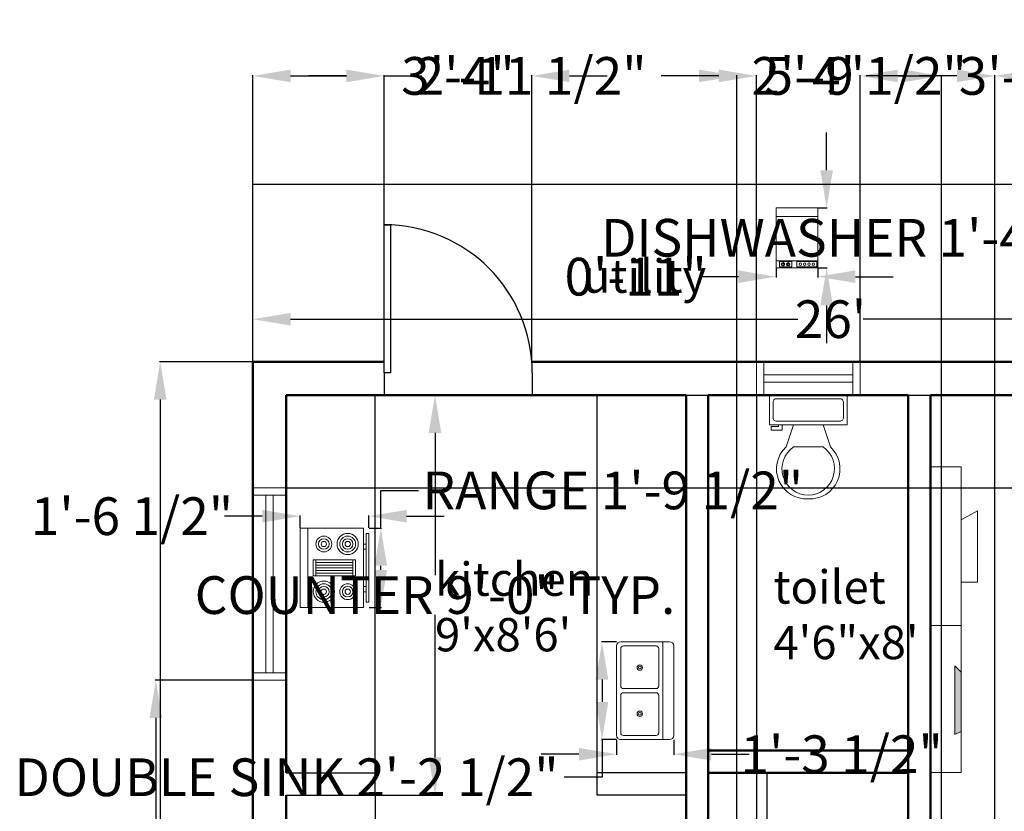
# Model space of a CAD drawing. Units: inches. Extents: x 20 to 3619, y 7 to 1288.
# Tile 3 of 4: x 3080 to 3346, y 1074 to 1288. Entities that reach past the tile are written whole.
import ezdxf

# ---------------------------------------------------------------- set-up
doc = ezdxf.new("R2010")
doc.units = ezdxf.units.IN
doc.header["$MEASUREMENT"] = 0
for name, color, linetype, lineweight in [('A-ANNO-DIMS', 2, 'Continuous', 18), ('A-AREA-IDEN', 7, 'Continuous', 25), ('A-DOOR', 3, 'Continuous', 25), ('A-EQPM', 8, 'Continuous', 18), ('A-FLOR-CASE', 9, 'Continuous', 25), ('A-FLOR-FIXT', 9, 'Continuous', 18), ('A-FURN', 8, 'Continuous', 18), ('A-GLAZ', 4, 'Continuous', 18), ('A-WALL', 7, 'Continuous', 50), ('C-PROP', 8, 'Continuous', 25)]:
    doc.layers.add(name, color=color, linetype=linetype, lineweight=lineweight)
doc.layers.add('A-FURN-PATT', color=18, linetype='Continuous', lineweight=13, true_color=0x000000)
doc.styles.get("Standard").update_dxf_attribs({"font": 'arial.ttf'})
doc.dimstyles.get("Standard").update_dxf_attribs({"dimtxt": 10.18, "dimasz": 10.18, "dimexe": 0.18, "dimexo": 0.0625, "dimgap": 0.09, "dimtad": 0, "dimtih": 1, "dimtoh": 1, "dimdec": 0, "dimzin": 0, "dimdsep": 46, "dimlunit": 3, "dimtxsty": 'Standard', "dimcen": 0.09, "dimadec": 0, "dimazin": 0, "dimtfac": 1, "dimtdec": 0, "dimtofl": 0, "dimtmove": 0, "dimatfit": 3, "dimfxl": 1, "dimtolj": 1, "dimtzin": 0, "dimarcsym": 0})

# ---------------------------------------------------------------- blocks, each defined once
blk = doc.blocks.new('*D3')
at = {"layer": 'A-ANNO-DIMS', "color": 0, "lineweight": -2, "transparency": 16777216}
for p, q in [((3142.72, 1195.76), (3142.72, 1207.38)), ((3454.72, 1195.76), (3454.72, 1207.38)), ((3152.9, 1207.2), (3289.9, 1207.2)), ((3444.54, 1207.2), (3307.53, 1207.2))]:
    blk.add_line(p, q, dxfattribs=at)
at = {"layer": 'A-ANNO-DIMS', "color": 0, "transparency": 16777216}
for points in [[(3152.9, 1208.9), (3152.9, 1205.5), (3142.72, 1207.2)], [(3444.54, 1208.9), (3444.54, 1205.5), (3454.72, 1207.2)]]:
    blk.add_solid(points, dxfattribs=at)
at = {"layer": 'Defpoints', "color": 0, "transparency": 16777216}
for p in [(3454.72, 1207.2), (3142.72, 1195.69), (3454.72, 1195.69)]:
    blk.add_point(p, dxfattribs=at)
at = {"layer": 'A-ANNO-DIMS', "color": 0, "transparency": 16777216, "insert": (3298.72, 1207.2), "char_height": 10.18, "attachment_point": 5}
blk.add_mtext("\\A1;26'", dxfattribs=at)
blk = doc.blocks.new('*D4')
at = {"layer": 'A-ANNO-DIMS', "color": 0, "lineweight": -2, "transparency": 16777216}
for p, q in [((3142.66, 1195.69), (3117.53, 1195.69)), ((3117.71, 1185.51), (3117.71, 996.98)), ((3117.71, 797.87), (3117.71, 986.4)), ((3142.66, 787.69), (3117.53, 787.69))]:
    blk.add_line(p, q, dxfattribs=at)
at = {"layer": 'A-ANNO-DIMS', "color": 0, "transparency": 16777216}
for points in [[(3116.01, 1185.51), (3119.4, 1185.51), (3117.71, 1195.69)], [(3116.01, 797.87), (3119.4, 797.87), (3117.71, 787.69)]]:
    blk.add_solid(points, dxfattribs=at)
at = {"layer": 'Defpoints', "color": 0, "transparency": 16777216}
for p in [(3117.71, 1195.69), (3142.72, 1195.69), (3142.72, 787.69)]:
    blk.add_point(p, dxfattribs=at)
at = {"layer": 'A-ANNO-DIMS', "color": 0, "transparency": 16777216, "insert": (3117.71, 991.69), "char_height": 10.18, "attachment_point": 5}
blk.add_mtext("\\A1;34'", dxfattribs=at)
blk = doc.blocks.new('*U15')
for p, q in [((9.5, -6), (9.5, -2)), ((-10, -8.5), (-8, -8.5)), ((-10, -9.5), (-10, -8.5)), ((-7, -9.5), (-10, -9.5)), ((-8, -8.5), (-8, -8)), ((-7, -8), (-7, -9.5)), ((-4, -8), (-6, -14)), ((4, -8), (6, -14)), ((4, -14), (-4, -14))]:
    blk.add_line(p, q)
blk.add_lwpolyline([(10.5, -8), (10.5, 0), (-10.5, 0), (-10.5, -8)], close=True)
for points in [[(-9.5, -2), (-9.5, -6)], [(8.5, -1), (-8.5, -1)], [(-8.5, -7), (8.5, -7)]]:
    blk.add_lwpolyline(points)
for centre, radius, start, end in [((-8.625, -1.875), 0.8839, 81.8699, 188.1301), ((8.625, -1.875), 0.8839, 351.8699, 98.1301), ((-8.625, -6.125), 0.8839, 171.869898, 278.1301), ((8.625, -6.125), 0.8839, 261.8699, 8.1301), ((-0.4772, -19.9188), 8.0953, 133.01722, 273.38), ((0.0374, -19.8731), 7.127, 124.50543, 269.7), ((-0.0373, -19.8731), 7.127, 270.3, 55.4946), ((0.4773, -19.9188), 8.0953, 266.62, 46.9828)]:
    blk.add_arc(centre, radius, start, end)
blk = doc.blocks.new('Sink-double - 36 in top')
for p, q in [((-18, -4), (18, -4)), ((-0.75, -18.5), (-0.75, -6.5)), ((0.75, -6.5), (0.75, -18.5))]:
    blk.add_line(p, q)
for points in [[(-16.5, 0), (16.5, 0)], [(-18, -19.5), (-18, -1.5)], [(18, -1.5), (18, -19.5)], [(-16.5, -18.5), (-16.5, -6.5)], [(-15.5, -5.5), (-1.75, -5.5)], [(1.75, -5.5), (15.5, -5.5)], [(16.5, -6.5), (16.5, -18.5)], [(16.5, -21), (-16.5, -21)], [(-1.75, -19.5), (-15.5, -19.5)], [(15.5, -19.5), (1.75, -19.5)]]:
    blk.add_lwpolyline(points)
for centre, radius in [((-8.5, -12.5), 1), ((-8.5, -12.5), 0.5), ((8.5, -12.5), 1), ((8.5, -12.5), 0.5)]:
    blk.add_circle(centre, radius)
for centre, radius, start, end in [((-16.5, -1.5), 1.5, 90, 180), ((16.5, -1.5), 1.5, 0, 90), ((-15.5, -6.5), 1, 90, 180), ((-1.75, -6.5), 1, 0, 90), ((1.75, -6.5), 1, 90, 180), ((15.5, -6.5), 1, 0, 90), ((-16.5, -19.5), 1.5, 180, 270), ((-15.5, -18.5), 1, 180, 270), ((-1.75, -18.5), 1, 270, 0), ((1.75, -18.5), 1, 180, 270), ((15.5, -18.5), 1, 270, 0), ((16.5, -19.5), 1.5, 270, 0)]:
    blk.add_arc(centre, radius, start, end)
blk = doc.blocks.new('Range-Oven - 30 in top')
for p, q in [((0, -3), (30, -3)), ((12, -6), (18, -6)), ((13, -20), (13, -6)), ((14, -6), (14, -20)), ((15, -20), (15, -6)), ((16, -6), (16, -20)), ((17, -20), (17, -6)), ((18, -20), (12, -20)), ((6, -24), (6, -25)), ((8, -25), (8, -24)), ((22, -25), (22, -24)), ((24, -24), (24, -25))]:
    blk.add_line(p, q)
for points in [[(0, -24), (0, 0), (30, 0), (30, -24)], [(12, -21), (12, -5), (18, -5), (18, -21)], [(2, -26), (2, -25), (28, -25), (28, -26)]]:
    blk.add_lwpolyline(points, close=True)
for centre, radius in [((6, -9), 4), ((6, -9), 3), ((6, -9), 2), ((24, -9), 3), ((24, -9), 2), ((6, -9), 1), ((24, -9), 1), ((24, -18), 4), ((6, -18), 3), ((6, -18), 2), ((6, -18), 1), ((24, -18), 3), ((24, -18), 2), ((24, -18), 1)]:
    blk.add_circle(centre, radius)
blk = doc.blocks.new('Dishwasher')
for p, q in [((24, 30.5), (0, 30.5)), ((16, 32.5), (16.75, 32.5)), ((16.5, 32), (16.2942, 31.7942)), ((16.3156, 33.1843), (16.5, 33)), ((17, 32.75), (17, 33.5)), ((17, 32.25), (17, 31.5)), ((18, 32.5), (17.25, 32.5)), ((17.5, 33), (17.6938, 33.1938)), ((17.7061, 31.7939), (17.5, 32)), ((19, 32.5), (19.75, 32.5)), ((19.5, 32), (19.2942, 31.7942)), ((19.3156, 33.1843), (19.5, 33)), ((20, 32.75), (20, 33.5)), ((20, 32.25), (20, 31.5)), ((21, 32.5), (20.25, 32.5)), ((20.5, 33), (20.6938, 33.1938)), ((20.7061, 31.7939), (20.5, 32)), ((0, 5), (24, 5))]:
    blk.add_line(p, q)
for points in [[(0, 0), (0, 34.5), (24, 34.5), (24, 0)], [(0.5, 31), (0.5, 34), (12, 34), (12, 31)], [(15, 31), (15, 34), (22, 34), (22, 31)]]:
    blk.add_lwpolyline(points, close=True)
for centre, radius in [((2.5, 32.5), 0.75), ((5, 32.5), 0.75), ((7.5, 32.5), 0.75), ((10, 32.5), 0.75), ((17, 32.5), 1), ((20, 32.5), 1)]:
    blk.add_circle(centre, radius)
blk = doc.blocks.new('*U2')
for p, q in [((0, 0), (0, -6)), ((40, 0), (40, -6))]:
    blk.add_line(p, q)
blk.add_lwpolyline([(0, 0), (0, 40), (1.75, 40), (1.75, 0)], close=True)
blk.add_arc((0, 0), 40, 0, 90)
blk = doc.blocks.new('WIN-48IN-PLAN')
for p, q in [((0, 0), (0, 9)), ((2, 0), (2, 9)), ((50, 0), (50, 9)), ((52, 0), (52, 9)), ((2, 5.5), (50, 5.5)), ((2, 3.5), (50, 3.5))]:
    blk.add_line(p, q)
blk = doc.blocks.new('COUNTER-24X108IN')
for p, q in [((24, 0), (24, 108)), ((0, 6), (24, 6)), ((0, 0), (24, 0))]:
    blk.add_line(p, q)
blk = doc.blocks.new('*D24')
at = {"layer": 'A-ANNO-DIMS', "color": 0, "lineweight": -2, "transparency": 16777216}
for p, q in [((3175.78, 1186.69), (3192.1, 1186.69)), ((3191.92, 1176.51), (3191.92, 1138.05)), ((3191.92, 1088.87), (3191.92, 1127.34)), ((3175.78, 1078.69), (3192.1, 1078.69))]:
    blk.add_line(p, q, dxfattribs=at)
at = {"layer": 'A-ANNO-DIMS', "color": 0, "transparency": 16777216}
for points in [[(3190.22, 1176.51), (3193.61, 1176.51), (3191.92, 1186.69)], [(3190.22, 1088.87), (3193.61, 1088.87), (3191.92, 1078.69)]]:
    blk.add_solid(points, dxfattribs=at)
at = {"layer": 'Defpoints', "color": 0, "transparency": 16777216}
for p in [(3175.72, 1186.69), (3191.92, 1186.69), (3175.72, 1078.69)]:
    blk.add_point(p, dxfattribs=at)
at = {"layer": 'A-ANNO-DIMS', "color": 0, "transparency": 16777216, "insert": (3191.92, 1132.69), "char_height": 10.18, "attachment_point": 5}
blk.add_mtext('\\A1;COUNTER 9\'-0" TYP.', dxfattribs=at)
blk = doc.blocks.new('*D25')
at = {"layer": 'A-ANNO-DIMS', "color": 0, "lineweight": -2, "transparency": 16777216}
for p, q in [((3151.72, 1078.63), (3151.72, 1062.31)), ((3175.72, 1078.63), (3175.72, 1062.31)), ((3161.9, 1062.49), (3165.54, 1062.49)), ((3175.72, 1062.49), (3185.9, 1062.49))]:
    blk.add_line(p, q, dxfattribs=at)
at = {"layer": 'A-ANNO-DIMS', "color": 0, "transparency": 16777216}
for points in [[(3161.9, 1064.19), (3161.9, 1060.8), (3151.72, 1062.49)], [(3165.54, 1064.19), (3165.54, 1060.8), (3175.72, 1062.49)]]:
    blk.add_solid(points, dxfattribs=at)
at = {"layer": 'Defpoints', "color": 0, "transparency": 16777216}
for p in [(3151.72, 1078.69), (3175.72, 1078.69), (3175.72, 1062.49)]:
    blk.add_point(p, dxfattribs=at)
at = {"layer": 'A-ANNO-DIMS', "color": 0, "transparency": 16777216, "insert": (3217.1, 1062.49), "char_height": 10.18, "attachment_point": 5}
blk.add_mtext('\\A1;2\'-0" TYP.', dxfattribs=at)
blk = doc.blocks.new('*D30')
at = {"layer": 'A-ANNO-DIMS', "color": 0, "lineweight": -2, "transparency": 16777216}
for p, q in [((3240.92, 1120.08), (3236.84, 1120.08)), ((3237.02, 1109.9), (3237.02, 1103.86)), ((3240.92, 1093.68), (3236.84, 1093.68)), ((3237.02, 1093.68), (3237.02, 1083.5)), ((3237.02, 1083.5), (3226.84, 1083.5))]:
    blk.add_line(p, q, dxfattribs=at)
at = {"layer": 'A-ANNO-DIMS', "color": 0, "transparency": 16777216}
for points in [[(3235.33, 1109.9), (3238.72, 1109.9), (3237.02, 1120.08)], [(3235.33, 1103.86), (3238.72, 1103.86), (3237.02, 1093.68)]]:
    blk.add_solid(points, dxfattribs=at)
at = {"layer": 'Defpoints', "color": 0, "transparency": 16777216}
for p in [(3240.98, 1120.08), (3237.02, 1093.68), (3240.98, 1093.68)]:
    blk.add_point(p, dxfattribs=at)
at = {"layer": 'A-ANNO-DIMS', "color": 0, "transparency": 16777216, "insert": (3151.83, 1083.5), "char_height": 10.18, "attachment_point": 5}
blk.add_mtext('\\A1;DOUBLE SINK 2\'-2 1/2"', dxfattribs=at)
blk = doc.blocks.new('*D31')
at = {"layer": 'A-ANNO-DIMS', "color": 0, "lineweight": -2, "transparency": 16777216}
for p, q in [((3240.98, 1093.61), (3240.98, 1089.54)), ((3256.38, 1093.61), (3256.38, 1089.54)), ((3230.8, 1089.72), (3220.62, 1089.72)), ((3266.56, 1089.72), (3276.74, 1089.72))]:
    blk.add_line(p, q, dxfattribs=at)
at = {"layer": 'A-ANNO-DIMS', "color": 0, "transparency": 16777216}
for points in [[(3230.8, 1091.41), (3230.8, 1088.02), (3240.98, 1089.72)], [(3266.56, 1091.41), (3266.56, 1088.02), (3256.38, 1089.72)]]:
    blk.add_solid(points, dxfattribs=at)
at = {"layer": 'Defpoints', "color": 0, "transparency": 16777216}
for p in [(3240.98, 1093.68), (3256.38, 1093.68), (3256.38, 1089.72)]:
    blk.add_point(p, dxfattribs=at)
at = {"layer": 'A-ANNO-DIMS', "color": 0, "transparency": 16777216, "insert": (3301.75, 1089.72), "char_height": 10.18, "attachment_point": 5}
blk.add_mtext('\\A1;1\'-3 1/2"', dxfattribs=at)
blk = doc.blocks.new('*D32')
at = {"layer": 'A-ANNO-DIMS', "color": 0, "lineweight": -2, "transparency": 16777216}
for p, q in [((3177.28, 1150.78), (3177.28, 1160.96)), ((3177.28, 1160.96), (3187.46, 1160.96)), ((3174.12, 1150.78), (3177.46, 1150.78)), ((3177.28, 1139.5), (3177.28, 1140.6)), ((3174.12, 1129.32), (3177.46, 1129.32))]:
    blk.add_line(p, q, dxfattribs=at)
at = {"layer": 'A-ANNO-DIMS', "color": 0, "transparency": 16777216}
for points in [[(3175.58, 1140.6), (3178.97, 1140.6), (3177.28, 1150.78)], [(3175.58, 1139.5), (3178.97, 1139.5), (3177.28, 1129.32)]]:
    blk.add_solid(points, dxfattribs=at)
at = {"layer": 'Defpoints', "color": 0, "transparency": 16777216}
for p in [(3174.06, 1150.78), (3177.28, 1150.78), (3174.06, 1129.32)]:
    blk.add_point(p, dxfattribs=at)
at = {"layer": 'A-ANNO-DIMS', "color": 0, "transparency": 16777216, "insert": (3239.94, 1160.96), "char_height": 10.18, "attachment_point": 5}
blk.add_mtext('\\A1;RANGE 1\'-9 1/2"', dxfattribs=at)
blk = doc.blocks.new('*D33')
at = {"layer": 'A-ANNO-DIMS', "color": 0, "lineweight": -2, "transparency": 16777216}
for p, q in [((3155.46, 1150.84), (3155.46, 1154.18)), ((3174.06, 1150.84), (3174.06, 1154.18)), ((3145.28, 1154), (3135.1, 1154)), ((3184.24, 1154), (3194.42, 1154))]:
    blk.add_line(p, q, dxfattribs=at)
at = {"layer": 'A-ANNO-DIMS', "color": 0, "transparency": 16777216}
for points in [[(3145.28, 1155.7), (3145.28, 1152.3), (3155.46, 1154)], [(3184.24, 1155.7), (3184.24, 1152.3), (3174.06, 1154)]]:
    blk.add_solid(points, dxfattribs=at)
at = {"layer": 'Defpoints', "color": 0, "transparency": 16777216}
for p in [(3155.46, 1154), (3155.46, 1150.78), (3174.06, 1150.78)]:
    blk.add_point(p, dxfattribs=at)
at = {"layer": 'A-ANNO-DIMS', "color": 0, "transparency": 16777216, "insert": (3110.09, 1154), "char_height": 10.18, "attachment_point": 5}
blk.add_mtext('\\A1;1\'-6 1/2"', dxfattribs=at)
blk = doc.blocks.new('*D34')
at = {"layer": 'A-ANNO-DIMS', "color": 0, "lineweight": -2, "transparency": 16777216}
for p, q in [((3297.69, 1247.43), (3297.69, 1257.61)), ((3295.33, 1237.25), (3297.87, 1237.25)), ((3295.33, 1221.1), (3297.87, 1221.1)), ((3297.69, 1210.92), (3297.69, 1200.74))]:
    blk.add_line(p, q, dxfattribs=at)
at = {"layer": 'A-ANNO-DIMS', "color": 0, "transparency": 16777216}
for points in [[(3295.99, 1247.43), (3299.38, 1247.43), (3297.69, 1237.25)], [(3295.99, 1210.92), (3299.38, 1210.92), (3297.69, 1221.1)]]:
    blk.add_solid(points, dxfattribs=at)
at = {"layer": 'Defpoints', "color": 0, "transparency": 16777216}
for p in [(3295.27, 1237.25), (3295.27, 1221.1), (3297.69, 1221.1)]:
    blk.add_point(p, dxfattribs=at)
at = {"layer": 'A-ANNO-DIMS', "color": 0, "transparency": 16777216, "insert": (3297.69, 1229.18), "char_height": 10.18, "attachment_point": 5}
blk.add_mtext('\\A1;DISHWASHER 1\'-4"', dxfattribs=at)
blk = doc.blocks.new('*D35')
at = {"layer": 'A-ANNO-DIMS', "color": 0, "lineweight": -2, "transparency": 16777216}
for p, q in [((3284.03, 1221.04), (3284.03, 1218.5)), ((3295.27, 1221.04), (3295.27, 1218.5)), ((3273.85, 1218.68), (3263.67, 1218.68)), ((3305.45, 1218.68), (3315.63, 1218.68))]:
    blk.add_line(p, q, dxfattribs=at)
at = {"layer": 'A-ANNO-DIMS', "color": 0, "transparency": 16777216}
for points in [[(3273.85, 1220.38), (3273.85, 1216.98), (3284.03, 1218.68)], [(3305.45, 1220.38), (3305.45, 1216.98), (3295.27, 1218.68)]]:
    blk.add_solid(points, dxfattribs=at)
at = {"layer": 'Defpoints', "color": 0, "transparency": 16777216}
for p in [(3284.03, 1221.1), (3295.27, 1221.1), (3284.03, 1218.68)]:
    blk.add_point(p, dxfattribs=at)
at = {"layer": 'A-ANNO-DIMS', "color": 0, "transparency": 16777216, "insert": (3246.1, 1218.68), "char_height": 10.18, "attachment_point": 5}
blk.add_mtext('\\A1;0\'-11"', dxfattribs=at)
blk = doc.blocks.new('*D38')
at = {"layer": 'A-ANNO-DIMS', "color": 0, "lineweight": -2, "transparency": 16777216}
for p, q in [((3142.72, 1195.76), (3142.72, 1273.07)), ((3152.9, 1272.89), (3168, 1272.89)), ((3178.18, 1195.76), (3178.18, 1273.07)), ((3178.18, 1272.89), (3188.36, 1272.89))]:
    blk.add_line(p, q, dxfattribs=at)
at = {"layer": 'A-ANNO-DIMS', "color": 0, "transparency": 16777216}
for points in [[(3152.9, 1274.59), (3152.9, 1271.2), (3142.72, 1272.89)], [(3168, 1274.59), (3168, 1271.2), (3178.18, 1272.89)]]:
    blk.add_solid(points, dxfattribs=at)
at = {"layer": 'Defpoints', "color": 0, "transparency": 16777216}
for p in [(3178.18, 1272.89), (3142.72, 1195.69), (3178.18, 1195.69)]:
    blk.add_point(p, dxfattribs=at)
at = {"layer": 'A-ANNO-DIMS', "color": 0, "transparency": 16777216, "insert": (3217.88, 1272.89), "char_height": 10.18, "attachment_point": 5}
blk.add_mtext('\\A1;2\'-11 1/2"', dxfattribs=at)
blk = doc.blocks.new('*D39')
at = {"layer": 'A-ANNO-DIMS', "color": 0, "lineweight": -2, "transparency": 16777216}
for p, q in [((3168, 1272.89), (3157.82, 1272.89)), ((3178.18, 1195.76), (3178.18, 1273.07)), ((3218.06, 1195.76), (3218.06, 1273.07)), ((3228.24, 1272.89), (3238.42, 1272.89))]:
    blk.add_line(p, q, dxfattribs=at)
at = {"layer": 'A-ANNO-DIMS', "color": 0, "transparency": 16777216}
for points in [[(3168, 1274.59), (3168, 1271.2), (3178.18, 1272.89)], [(3228.24, 1274.59), (3228.24, 1271.2), (3218.06, 1272.89)]]:
    blk.add_solid(points, dxfattribs=at)
at = {"layer": 'Defpoints', "color": 0, "transparency": 16777216}
for p in [(3218.06, 1272.89), (3178.18, 1195.69), (3218.06, 1195.69)]:
    blk.add_point(p, dxfattribs=at)
at = {"layer": 'A-ANNO-DIMS', "color": 0, "transparency": 16777216, "insert": (3198.12, 1272.89), "char_height": 10.18, "attachment_point": 5}
blk.add_mtext('\\A1;3\'-4"', dxfattribs=at)
blk = doc.blocks.new('*D40')
at = {"layer": 'A-ANNO-DIMS', "color": 0, "lineweight": -2, "transparency": 16777216}
for p, q in [((3332.89, 1272.89), (3322.71, 1272.89)), ((3343.07, 796.76), (3343.07, 1273.07)), ((3382.22, 796.76), (3382.22, 1273.07)), ((3392.4, 1272.89), (3402.58, 1272.89))]:
    blk.add_line(p, q, dxfattribs=at)
at = {"layer": 'A-ANNO-DIMS', "color": 0, "transparency": 16777216}
for points in [[(3332.89, 1274.59), (3332.89, 1271.2), (3343.07, 1272.89)], [(3392.4, 1274.59), (3392.4, 1271.2), (3382.22, 1272.89)]]:
    blk.add_solid(points, dxfattribs=at)
at = {"layer": 'Defpoints', "color": 0, "transparency": 16777216}
for p in [(3382.22, 1272.89), (3343.07, 796.69), (3382.22, 796.69)]:
    blk.add_point(p, dxfattribs=at)
at = {"layer": 'A-ANNO-DIMS', "color": 0, "transparency": 16777216, "insert": (3362.64, 1272.89), "char_height": 10.18, "attachment_point": 5}
blk.add_mtext('\\A1;3\'-3"', dxfattribs=at)
blk = doc.blocks.new('*D41')
at = {"layer": 'A-ANNO-DIMS', "color": 0, "lineweight": -2, "transparency": 16777216}
for p, q in [((3263.21, 1272.89), (3253.03, 1272.89)), ((3273.39, 796.76), (3273.39, 1273.07)), ((3343.07, 796.76), (3343.07, 1273.07)), ((3353.25, 1272.89), (3363.43, 1272.89))]:
    blk.add_line(p, q, dxfattribs=at)
at = {"layer": 'A-ANNO-DIMS', "color": 0, "transparency": 16777216}
for points in [[(3263.21, 1274.59), (3263.21, 1271.2), (3273.39, 1272.89)], [(3353.25, 1274.59), (3353.25, 1271.2), (3343.07, 1272.89)]]:
    blk.add_solid(points, dxfattribs=at)
at = {"layer": 'Defpoints', "color": 0, "transparency": 16777216}
for p in [(3343.07, 1272.89), (3273.39, 796.69), (3343.07, 796.69)]:
    blk.add_point(p, dxfattribs=at)
at = {"layer": 'A-ANNO-DIMS', "color": 0, "transparency": 16777216, "insert": (3308.23, 1272.89), "char_height": 10.18, "attachment_point": 5}
blk.add_mtext('\\A1;5\'-9 1/2"', dxfattribs=at)
blk = doc.blocks.new('*D43')
at = {"layer": 'A-ANNO-DIMS', "color": 0, "lineweight": -2, "transparency": 16777216}
for p, q in [((3142.66, 1109.69), (3116.34, 1109.69)), ((3116.52, 1099.51), (3116.52, 1064.93)), ((3116.52, 1019.77), (3116.52, 1054.35)), ((3142.66, 1009.59), (3116.34, 1009.59))]:
    blk.add_line(p, q, dxfattribs=at)
at = {"layer": 'A-ANNO-DIMS', "color": 0, "transparency": 16777216}
for points in [[(3114.82, 1099.51), (3118.21, 1099.51), (3116.52, 1109.69)], [(3114.82, 1019.77), (3118.21, 1019.77), (3116.52, 1009.59)]]:
    blk.add_solid(points, dxfattribs=at)
at = {"layer": 'Defpoints', "color": 0, "transparency": 16777216}
for p in [(3116.52, 1109.69), (3142.72, 1109.69), (3142.72, 1009.59)]:
    blk.add_point(p, dxfattribs=at)
at = {"layer": 'A-ANNO-DIMS', "color": 0, "transparency": 16777216, "insert": (3116.52, 1059.64), "char_height": 10.18, "attachment_point": 5}
blk.add_mtext('\\A1;8\'-4"', dxfattribs=at)
blk = doc.blocks.new('*D44')
at = {"layer": 'A-ANNO-DIMS', "color": 0, "lineweight": -2, "transparency": 16777216}
for p, q in [((3540.92, 1186.69), (3540.92, 1196.87)), ((3540.92, 1196.87), (3551.1, 1196.87)), ((3151.78, 1186.69), (3541.1, 1186.69)), ((3540.92, 1171.87), (3540.92, 1176.51)), ((3151.78, 1161.69), (3541.1, 1161.69))]:
    blk.add_line(p, q, dxfattribs=at)
at = {"layer": 'A-ANNO-DIMS', "color": 0, "transparency": 16777216}
for points in [[(3539.22, 1176.51), (3542.61, 1176.51), (3540.92, 1186.69)], [(3539.22, 1171.87), (3542.61, 1171.87), (3540.92, 1161.69)]]:
    blk.add_solid(points, dxfattribs=at)
at = {"layer": 'Defpoints', "color": 0, "transparency": 16777216}
for p in [(3151.72, 1186.69), (3540.92, 1186.69), (3151.72, 1161.69)]:
    blk.add_point(p, dxfattribs=at)
at = {"layer": 'A-ANNO-DIMS', "color": 0, "transparency": 16777216, "insert": (3564.81, 1196.87), "char_height": 10.18, "attachment_point": 5}
blk.add_mtext('\\A1;2\'-1"', dxfattribs=at)
blk = doc.blocks.new('*D46')
at = {"layer": 'A-ANNO-DIMS', "color": 0, "lineweight": -2, "transparency": 16777216}
for p, q in [((3268.54, 1272.89), (3258.36, 1272.89)), ((3278.72, 1195.76), (3278.72, 1273.07)), ((3306.72, 1195.76), (3306.72, 1273.07)), ((3316.9, 1272.89), (3327.08, 1272.89))]:
    blk.add_line(p, q, dxfattribs=at)
at = {"layer": 'A-ANNO-DIMS', "color": 0, "transparency": 16777216}
for points in [[(3268.54, 1274.59), (3268.54, 1271.2), (3278.72, 1272.89)], [(3316.9, 1274.59), (3316.9, 1271.2), (3306.72, 1272.89)]]:
    blk.add_solid(points, dxfattribs=at)
at = {"layer": 'Defpoints', "color": 0, "transparency": 16777216}
for p in [(3306.72, 1272.89), (3278.72, 1195.69), (3306.72, 1195.69)]:
    blk.add_point(p, dxfattribs=at)
at = {"layer": 'A-ANNO-DIMS', "color": 0, "transparency": 16777216, "insert": (3292.72, 1272.89), "char_height": 10.18, "attachment_point": 5}
blk.add_mtext('\\A1;2\'-4"', dxfattribs=at)
blk = doc.blocks.new('*D47')
at = {"layer": 'A-ANNO-DIMS', "color": 0, "lineweight": -2, "transparency": 16777216}
for p, q in [((3265.72, 1186.63), (3265.72, 701.31)), ((3278.72, 1186.63), (3278.72, 701.31)), ((3255.54, 701.49), (3245.36, 701.49)), ((3288.9, 701.49), (3299.08, 701.49))]:
    blk.add_line(p, q, dxfattribs=at)
at = {"layer": 'A-ANNO-DIMS', "color": 0, "transparency": 16777216}
for points in [[(3255.54, 703.19), (3255.54, 699.8), (3265.72, 701.49)], [(3288.9, 703.19), (3288.9, 699.8), (3278.72, 701.49)]]:
    blk.add_solid(points, dxfattribs=at)
at = {"layer": 'Defpoints', "color": 0, "transparency": 16777216}
for p in [(3265.72, 1186.69), (3278.72, 1186.69), (3278.72, 701.49)]:
    blk.add_point(p, dxfattribs=at)
at = {"layer": 'A-ANNO-DIMS', "color": 0, "transparency": 16777216, "insert": (3312.22, 701.49), "char_height": 10.18, "attachment_point": 5}
blk.add_mtext('\\A1;1\'-1"', dxfattribs=at)
blk = doc.blocks.new('*D52')
at = {"layer": 'A-ANNO-DIMS', "color": 0, "lineweight": -2, "transparency": 16777216}
for p, q in [((3318.54, 1272.89), (3308.36, 1272.89)), ((3328.72, 1018.76), (3328.72, 1273.07)), ((3368.72, 1018.76), (3368.72, 1273.07)), ((3378.9, 1272.89), (3389.08, 1272.89))]:
    blk.add_line(p, q, dxfattribs=at)
at = {"layer": 'A-ANNO-DIMS', "color": 0, "transparency": 16777216}
for points in [[(3318.54, 1274.59), (3318.54, 1271.2), (3328.72, 1272.89)], [(3378.9, 1274.59), (3378.9, 1271.2), (3368.72, 1272.89)]]:
    blk.add_solid(points, dxfattribs=at)
at = {"layer": 'Defpoints', "color": 0, "transparency": 16777216}
for p in [(3368.72, 1272.89), (3328.72, 1018.69), (3368.72, 1018.69)]:
    blk.add_point(p, dxfattribs=at)
at = {"layer": 'A-ANNO-DIMS', "color": 0, "transparency": 16777216, "insert": (3348.72, 1272.89), "char_height": 10.18, "attachment_point": 5}
blk.add_mtext('\\A1;3\'-4"', dxfattribs=at)

msp = doc.modelspace()

# ---------------------------------------------------------------- hatches: boundary and pattern name
at = {"layer": 'A-FURN-PATT'}
h = msp.add_hatch(color=256, dxfattribs=at)
h.dxf.hatch_style = 1
h.paths.add_polyline_path([(3334.05, 1111.87), (3332.28, 1113.61), (3332.28, 1095.07), (3334.05, 1095.82)])

# ---------------------------------------------------------------- linework, layer by layer
at = {"layer": 'A-FLOR-CASE'}
msp.add_line((3281.56, 1084.69), (3281.56, 1043.99), dxfattribs=at)
at = {"layer": 'A-FURN'}
for p, q in [((3334.05, 1167.33), (3325.72, 1167.33)), ((3334.05, 1153.02), (3338.44, 1155.47)), ((3338.44, 1155.47), (3338.44, 1136.2)), ((3338.44, 1136.2), (3334.05, 1136.2)), ((3334.05, 1111.87), (3332.28, 1113.61)), ((3332.28, 1113.61), (3332.28, 1095.07)), ((3332.28, 1095.07), (3334.05, 1095.82))]:
    msp.add_line(p, q, dxfattribs=at)
for points in [[(3334.05, 1124.45), (3334.05, 1124.45), (3334.05, 1167.33), (3334.05, 1167.33)], [(3325.72, 1124.45), (3334.05, 1124.45), (3334.05, 1084.78), (3325.72, 1084.78)]]:
    msp.add_lwpolyline(points, close=True, dxfattribs=at)
at = {"layer": 'A-GLAZ'}
for p, q in [((3278.72, 1186.69), (3278.72, 1195.69)), ((3280.72, 1186.69), (3280.72, 1195.69)), ((3304.72, 1186.69), (3304.72, 1195.69)), ((3306.72, 1186.69), (3306.72, 1195.69)), ((3280.72, 1192.19), (3304.72, 1192.19)), ((3280.72, 1190.19), (3304.72, 1190.19)), ((3148.22, 1159.69), (3148.22, 1111.69)), ((3148.22, 1159.69), (3148.22, 1111.69))]:
    msp.add_line(p, q, dxfattribs=at)
at = {"layer": 'A-WALL'}
for p, q in [((3142.72, 787.69), (3142.72, 1195.69)), ((3142.72, 1195.69), (3178.18, 1195.69)), ((3218.06, 1195.69), (3454.72, 1195.69)), ((3151.72, 1186.69), (3259.72, 1186.69)), ((3151.72, 1084.69), (3151.72, 1186.69)), ((3259.72, 1078.69), (3259.72, 1186.69)), ((3265.72, 1078.69), (3265.72, 1186.69)), ((3265.72, 1186.69), (3319.72, 1186.69)), ((3319.72, 1012.69), (3319.72, 1186.69)), ((3319.72, 1012.69), (3319.72, 1186.69)), ((3325.72, 1018.69), (3325.72, 1186.69)), ((3325.72, 1186.69), (3445.72, 1186.69)), ((3265.72, 1090.69), (3319.72, 1090.69)), ((3265.72, 1078.69), (3265.72, 1084.69)), ((3265.72, 1084.69), (3319.72, 1084.69)), ((3151.72, 796.69), (3151.72, 1078.69)), ((3259.72, 1078.69), (3259.72, 1037.99)), ((3265.72, 1078.69), (3265.72, 1043.99))]:
    msp.add_line(p, q, dxfattribs=at)
at = {"layer": 'C-PROP'}
for p, q in [((3142.72, 1243.69), (3514.72, 1243.69)), ((3142.72, 1195.69), (3142.72, 1243.69))]:
    msp.add_line(p, q, dxfattribs=at)

# ---------------------------------------------------------------- block references
at = {"layer": 'A-DOOR'}
msp.add_blockref('*U2', (3178.18, 1192.69), dxfattribs=at)
at = {"layer": 'A-EQPM'}
for name, p, xscale, yscale, zscale, rotation in [('Dishwasher', (3295.27, 1237.25), 0.4680781646985249, 0.4680781646985249, 0.4680781646985249, 180), ('Range-Oven - 30 in top', (3155.46, 1129.32), 0.7154257868435061, 0.7154257868435061, 0.7154257868435061, 90)]:
    msp.add_blockref(name, p, dxfattribs=dict(at, xscale=xscale, yscale=yscale, zscale=zscale, rotation=rotation))
at = {"layer": 'A-FLOR-CASE'}
msp.add_blockref('COUNTER-24X108IN', (3151.72, 1078.69), dxfattribs=at)
at = {"layer": 'A-FLOR-CASE', "extrusion": (0, 0, -1), "zscale": -1}
msp.add_blockref('COUNTER-24X108IN', (-3259.72, 1078.69), dxfattribs=at)
at = {"layer": 'A-FLOR-FIXT'}
msp.add_blockref('*U15', (3292.72, 1186.69), dxfattribs=at)
at = {"layer": 'A-FLOR-FIXT', "xscale": 0.7333233437057767, "yscale": 0.7333233437057767, "zscale": 0.7333233437057767, "rotation": 270}
msp.add_blockref('Sink-double - 36 in top', (3256.38, 1106.88), dxfattribs=at)
at = {"layer": 'A-GLAZ', "rotation": 270.0000000000002}
msp.add_blockref('WIN-48IN-PLAN', (3142.72, 1161.69), dxfattribs=at)

# ---------------------------------------------------------------- texts
at = {"layer": 'A-AREA-IDEN', "char_height": 9, "attachment_point": 1}
for s, insert in [('utility', (3231.82, 1223.34)), ("kitchen\\P9'x8'6' ", (3191.92, 1141.5)), ('toilet\\P4\'6"x8\' ', (3283.31, 1139.39))]:
    msp.add_mtext_dynamic_manual_height_columns(s, width=17.3739, gutter_width=1, heights=[0], dxfattribs=dict(at, insert=insert))

# ---------------------------------------------------------------- dimensions: what is measured, and where the dimension line sits
at = {"layer": 'A-ANNO-DIMS'}
for base, p1, p2, override, picture, middle in [((3178.18, 1272.89), (3142.72, 1195.69), (3178.18, 1195.69), {"dimdec": 1, "dimlfac": 1, "dimrnd": 0, "dimzin": 1, "dimdsep": 46, "dimlunit": 4, "dimfrac": 2}, '*D38', (3217.88, 1272.89)), ((3343.07, 1272.89), (3273.39, 796.69), (3343.07, 796.69), {"dimdec": 1, "dimlfac": 1, "dimrnd": 0, "dimzin": 1, "dimdsep": 46, "dimlunit": 4, "dimfrac": 2}, '*D41', (3308.23, 1272.89)), ((3218.06, 1272.89), (3178.18, 1195.69), (3218.06, 1195.69), {"dimdec": 1, "dimlfac": 1, "dimrnd": 0, "dimzin": 1, "dimdsep": 46, "dimlunit": 4, "dimfrac": 2}, '*D39', (3198.12, 1272.89)), ((3306.72, 1272.89), (3278.72, 1195.69), (3306.72, 1195.69), {"dimdec": 1, "dimlfac": 1, "dimrnd": 0, "dimzin": 1, "dimdsep": 46, "dimlunit": 4, "dimfrac": 2}, '*D46', (3292.72, 1272.89)), ((3368.72, 1272.89), (3328.72, 1018.69), (3368.72, 1018.69), {"dimdec": 1, "dimlfac": 1, "dimrnd": 0, "dimzin": 1, "dimdsep": 46, "dimlunit": 4, "dimfrac": 2}, '*D52', (3348.72, 1272.89)), ((3382.2188, 1272.8933), (3343.0711, 796.6933), (3382.2188, 796.6933), {"dimdec": 1, "dimlfac": 1, "dimrnd": 0, "dimzin": 1, "dimdsep": 46, "dimlunit": 4, "dimfrac": 2}, '*D40', (3362.6449, 1272.8933)), ((3454.72, 1207.2), (3142.72, 1195.69), (3454.72, 1195.69), {"dimclrd": 0, "dimclre": 0, "dimclrt": 0}, '*D3', (3298.72, 1207.2)), ((3278.72, 701.49), (3265.72, 1186.69), (3278.72, 1186.69), {"dimdec": 1, "dimlfac": 1, "dimrnd": 0, "dimzin": 1, "dimdsep": 46, "dimlunit": 4, "dimfrac": 2}, '*D47', (3312.22, 701.49)), ((3256.38, 1089.72), (3240.98, 1093.68), (3256.38, 1093.68), {"dimdec": 1, "dimlfac": 1, "dimrnd": 0, "dimzin": 1, "dimdsep": 46, "dimlunit": 4, "dimfrac": 2}, '*D31', (3301.75, 1089.72))]:
    dim = msp.add_linear_dim(base=base, p1=p1, p2=p2, dimstyle='Standard', override=override, dxfattribs=at)
    dim.commit()
    dim.dimension.update_dxf_attribs({"geometry": picture, "text_midpoint": middle})
for base, p1, p2, angle, text, picture, middle in [((3297.6875, 1221.1016), (3295.2652, 1237.2503), (3295.2652, 1221.1016), 270, 'DISHWASHER <>', '*D34', (3297.6875, 1229.1759)), ((3191.92, 1186.69), (3175.72, 1078.69), (3175.72, 1186.69), 90, 'COUNTER <> TYP.', '*D24', (3191.92, 1132.69)), ((3177.28, 1150.78), (3174.06, 1129.32), (3174.06, 1150.78), 90, 'RANGE <>', '*D32', (3239.94, 1160.96)), ((3237.02, 1093.68), (3240.98, 1120.08), (3240.98, 1093.68), 270, 'DOUBLE SINK <>', '*D30', (3151.83, 1083.5))]:
    dim = msp.add_linear_dim(base=base, p1=p1, p2=p2, angle=angle, text=text, dimstyle='Standard', override={"dimdec": 1, "dimlfac": 1, "dimrnd": 0, "dimzin": 1, "dimdsep": 46, "dimlunit": 4, "dimfrac": 2}, dxfattribs=at)
    dim.commit()
    dim.dimension.update_dxf_attribs({"geometry": picture, "text_midpoint": middle})
for base, p1, p2, angle, override, picture, middle in [((3284.03, 1218.68), (3295.27, 1221.1), (3284.03, 1221.1), 180, {"dimdec": 1, "dimlfac": 1, "dimrnd": 0, "dimzin": 1, "dimdsep": 46, "dimlunit": 4, "dimfrac": 2}, '*D35', (3246.1, 1218.68)), ((3540.92, 1186.69), (3151.72, 1161.69), (3151.72, 1186.69), 90, {"dimdec": 1, "dimlfac": 1, "dimrnd": 0, "dimzin": 1, "dimdsep": 46, "dimlunit": 4, "dimfrac": 2}, '*D44', (3564.81, 1196.87)), ((3117.71, 1195.69), (3142.72, 787.69), (3142.72, 1195.69), 90, {"dimclrd": 0, "dimclre": 0, "dimclrt": 0}, '*D4', (3117.71, 991.69)), ((3155.46, 1154), (3174.06, 1150.78), (3155.46, 1150.78), 180, {"dimdec": 1, "dimlfac": 1, "dimrnd": 0, "dimzin": 1, "dimdsep": 46, "dimlunit": 4, "dimfrac": 2}, '*D33', (3110.09, 1154)), ((3116.52, 1109.69), (3142.72, 1009.59), (3142.72, 1109.69), 90, {"dimdec": 1, "dimlfac": 1, "dimrnd": 0, "dimzin": 1, "dimdsep": 46, "dimlunit": 4, "dimfrac": 2}, '*D43', (3116.52, 1059.64))]:
    dim = msp.add_linear_dim(base=base, p1=p1, p2=p2, angle=angle, dimstyle='Standard', override=override, dxfattribs=at)
    dim.commit()
    dim.dimension.update_dxf_attribs({"geometry": picture, "text_midpoint": middle})
dim = msp.add_linear_dim(base=(3175.72, 1062.49), p1=(3151.72, 1078.69), p2=(3175.72, 1078.69), text='<> TYP.', dimstyle='Standard', override={"dimdec": 1, "dimlfac": 1, "dimrnd": 0, "dimzin": 1, "dimdsep": 46, "dimlunit": 4, "dimfrac": 2}, dxfattribs=at)
dim.commit()
dim.dimension.update_dxf_attribs({"geometry": '*D25', "text_midpoint": (3217.1, 1062.49)})

doc.saveas('drawing.dxf')
